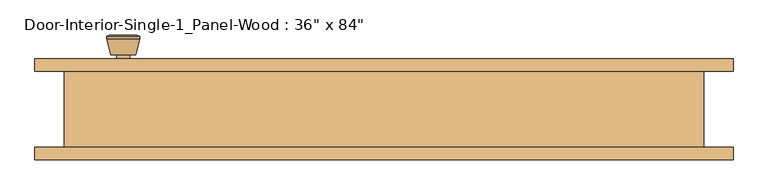
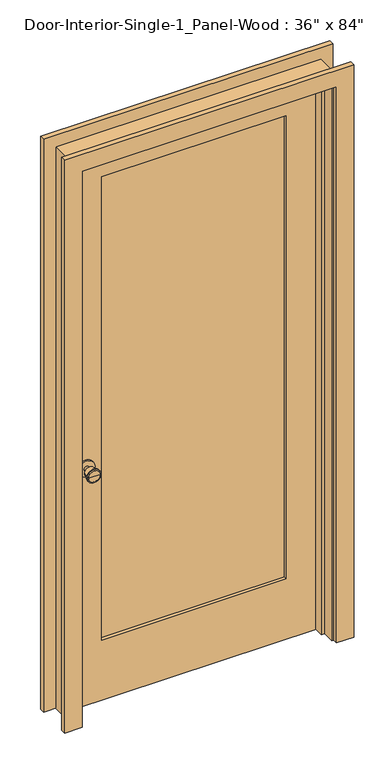
"""IFC4 building model written with IfcOpenShell, lengths in millimetres: door geometry."""

from ifc_helpers import new_model, si_unit, point, frame, frame_2d, origin, place, context, project, spatial, polyline, circle_curve, trimmed, segment, composite_curve, outline, extrude, faceted_brep, source, transform, mapped, element, save
from ifc_brep_helpers import plane_surface, cylinder_surface, revolved_surface, advanced_brep


def door_3c6ab76a(model_context):
    return source(origin(), model_context, "Body", "SolidModel", [
        advanced_brep(
        [(-393.7, 13.05, 914.4), (-383.7, 13.05, 914.4), (-403.7, 13.05, 914.4), (-373.2241324, -35.95, 914.4), (-393.7, -35.95, 914.4), (-414.1758676, -35.95, 914.4), (-368.7, -34.1221319, 914.4), (-418.7, -34.1221319, 914.4), (-368.7, -30.6584537, 914.4), (-418.7, -30.6584537, 914.4), (-375.063764, -5.95, 914.4), (-412.336236, -5.95, 914.4), (-383.7, -5.95, 914.4), (-403.7, -5.95, 914.4)],
        [
            (0, 1),
            (1, 2, circle_curve(frame((-393.7, 13.05, 914.4), z_axis=(0.0, 1.0, 0.0), x_axis=(-1.0, 0.0, 0.0)), 10.0)),
            (2, 0),
            (2, 1, circle_curve(frame((-393.7, 13.05, 914.4), z_axis=(0.0, 1.0, 0.0), x_axis=(-1.0, 0.0, 0.0)), 10.0)),
            (3, 4),
            (4, 5),
            (5, 3, circle_curve(frame((-393.7, -35.95, 914.4), z_axis=(0.0, -1.0, 0.0), x_axis=(-1.0, 0.0, 0.0)), 20.4758676)),
            (3, 5, circle_curve(frame((-393.7, -35.95, 914.4), z_axis=(0.0, -1.0, 0.0), x_axis=(-1.0, 0.0, 0.0)), 20.4758676)),
            (6, 3),
            (5, 7),
            (7, 6, circle_curve(frame((-393.7, -34.1221319, 914.4), z_axis=(0.0, -1.0, 0.0), x_axis=(-1.0, 0.0, 0.0)), 25.0)),
            (6, 7, circle_curve(frame((-393.7, -34.1221319, 914.4), z_axis=(0.0, -1.0, 0.0), x_axis=(-1.0, 0.0, 0.0)), 25.0)),
            (8, 6),
            (7, 9),
            (9, 8, circle_curve(frame((-393.7, -30.6584537, 914.4), z_axis=(0.0, -1.0, 0.0), x_axis=(-1.0, 0.0, 0.0)), 25.0)),
            (8, 9, circle_curve(frame((-393.7, -30.6584537, 914.4), z_axis=(0.0, -1.0, 0.0), x_axis=(-1.0, 0.0, 0.0)), 25.0)),
            (10, 8),
            (9, 11),
            (11, 10, circle_curve(frame((-393.7, -5.95, 914.4), z_axis=(0.0, -1.0, 0.0), x_axis=(-1.0, 0.0, 0.0)), 18.636236)),
            (10, 11, circle_curve(frame((-393.7, -5.95, 914.4), z_axis=(0.0, -1.0, 0.0), x_axis=(-1.0, 0.0, 0.0)), 18.636236)),
            (12, 10),
            (11, 13),
            (13, 12, circle_curve(frame((-393.7, -5.95, 914.4), z_axis=(0.0, -1.0, 0.0), x_axis=(-1.0, 0.0, 0.0)), 10.0)),
            (12, 13, circle_curve(frame((-393.7, -5.95, 914.4), z_axis=(0.0, -1.0, 0.0), x_axis=(-1.0, 0.0, 0.0)), 10.0)),
            (1, 12),
            (13, 2),
        ],
        [
            plane_surface(frame((-393.7, 13.05, 914.4), z_axis=(0.0, 1.0, 0.0), x_axis=(-1.0, 0.0, 0.0))),
            plane_surface(frame((-393.7, -35.95, 914.4), z_axis=(0.0, -1.0, 0.0), x_axis=(-1.0, 0.0, 0.0))),
            revolved_surface(polyline([(-414.1758676, -35.95, 914.4), (-418.7, -34.1221319, 914.4)]), (-393.7, 13.05, 914.4), (0.0, 1.0, 0.0)),
            cylinder_surface(frame((-393.7, 13.05, 914.4), z_axis=(0.0, 1.0, 0.0), x_axis=(-1.0, 0.0, 0.0)), 25.0),
            revolved_surface(polyline([(-418.7, -30.6584537, 914.4), (-412.336236, -5.95, 914.4)]), (-393.7, 13.05, 914.4), (0.0, 1.0, 0.0)),
            plane_surface(frame((-393.7, -5.95, 914.4), z_axis=(0.0, 1.0, 0.0), x_axis=(-1.0, 0.0, 0.0))),
            cylinder_surface(frame((-393.7, 13.05, 914.4), z_axis=(0.0, 1.0, 0.0), x_axis=(-1.0, 0.0, 0.0)), 10.0),
        ],
        [
            (0, [[1, 2, 3]]),
            (0, [[-3, 4, -1]]),
            (1, [[5, 6, 7]]),
            (1, [[-6, -5, 8]]),
            (2, [[9, -7, 10, 11]]),
            (2, [[-10, -8, -9, 12]]),
            (3, [[13, -11, 14, 15]]),
            (3, [[-14, -12, -13, 16]]),
            (4, [[17, -15, 18, 19]]),
            (4, [[-18, -16, -17, 20]]),
            (5, [[21, -19, 22, 23]]),
            (5, [[-22, -20, -21, 24]]),
            (6, [[25, -23, 26, -2]]),
            (6, [[-26, -24, -25, -4]]),
        ],
    ),
        extrude(outline(composite_curve([segment(trimmed(circle_curve(frame_2d((914.4, -393.7)), 30.0), [point((914.4, -423.7))], [point((914.4, -363.7))], False, "CARTESIAN"), True, "CONTINUOUS"), segment(trimmed(circle_curve(frame_2d((914.4, -393.7)), 30.0), [point((914.4, -363.7))], [point((914.4, -423.7))], False, "CARTESIAN"), True, "CONTINUOUS")], self_intersect=False)), frame((0.0, 13.05, 0.0), z_axis=(0.0, 1.0, 0.0), x_axis=(0.0, 0.0, 1.0)), (0.0, 0.0, 1.0), 6.0),
        advanced_brep(
        [(-393.7, 59.975, 914.4), (-403.7, 59.975, 914.4), (-383.7, 59.975, 914.4), (-373.2241324, 108.975, 914.4), (-414.1758676, 108.975, 914.4), (-393.7, 108.975, 914.4), (-368.7, 107.1471319, 914.4), (-418.7, 107.1471319, 914.4), (-368.7, 103.6834537, 914.4), (-418.7, 103.6834537, 914.4), (-375.063764, 78.975, 914.4), (-412.336236, 78.975, 914.4), (-383.7, 78.975, 914.4), (-403.7, 78.975, 914.4)],
        [
            (0, 1),
            (1, 2, circle_curve(frame((-393.7, 59.975, 914.4), z_axis=(0.0, -1.0, 0.0), x_axis=(-1.0, 0.0, 0.0)), 10.0)),
            (2, 0),
            (2, 1, circle_curve(frame((-393.7, 59.975, 914.4), z_axis=(0.0, -1.0, 0.0), x_axis=(-1.0, 0.0, 0.0)), 10.0)),
            (3, 4, circle_curve(frame((-393.7, 108.975, 914.4), z_axis=(0.0, 1.0, 0.0), x_axis=(-1.0, 0.0, 0.0)), 20.4758676)),
            (4, 5),
            (5, 3),
            (4, 3, circle_curve(frame((-393.7, 108.975, 914.4), z_axis=(0.0, 1.0, 0.0), x_axis=(-1.0, 0.0, 0.0)), 20.4758676)),
            (6, 7, circle_curve(frame((-393.7, 107.1471319, 914.4), z_axis=(0.0, 1.0, 0.0), x_axis=(-1.0, 0.0, 0.0)), 25.0)),
            (7, 4),
            (3, 6),
            (7, 6, circle_curve(frame((-393.7, 107.1471319, 914.4), z_axis=(0.0, 1.0, 0.0), x_axis=(-1.0, 0.0, 0.0)), 25.0)),
            (8, 9, circle_curve(frame((-393.7, 103.6834537, 914.4), z_axis=(0.0, 1.0, 0.0), x_axis=(-1.0, 0.0, 0.0)), 25.0)),
            (9, 7),
            (6, 8),
            (9, 8, circle_curve(frame((-393.7, 103.6834537, 914.4), z_axis=(0.0, 1.0, 0.0), x_axis=(-1.0, 0.0, 0.0)), 25.0)),
            (10, 11, circle_curve(frame((-393.7, 78.975, 914.4), z_axis=(0.0, 1.0, 0.0), x_axis=(-1.0, 0.0, 0.0)), 18.636236)),
            (11, 9),
            (8, 10),
            (11, 10, circle_curve(frame((-393.7, 78.975, 914.4), z_axis=(0.0, 1.0, 0.0), x_axis=(-1.0, 0.0, 0.0)), 18.636236)),
            (12, 13, circle_curve(frame((-393.7, 78.975, 914.4), z_axis=(0.0, 1.0, 0.0), x_axis=(-1.0, 0.0, 0.0)), 10.0)),
            (13, 11),
            (10, 12),
            (13, 12, circle_curve(frame((-393.7, 78.975, 914.4), z_axis=(0.0, 1.0, 0.0), x_axis=(-1.0, 0.0, 0.0)), 10.0)),
            (1, 13),
            (12, 2),
        ],
        [
            plane_surface(frame((-393.7, 59.975, 914.4), z_axis=(0.0, -1.0, 0.0), x_axis=(-1.0, 0.0, 0.0))),
            plane_surface(frame((-393.7, 108.975, 914.4), z_axis=(0.0, 1.0, 0.0), x_axis=(-1.0, 0.0, 0.0))),
            revolved_surface(polyline([(-414.1758676, 108.975, 914.4), (-418.7, 107.1471319, 914.4)]), (-393.7, 59.975, 914.4), (0.0, -1.0, 0.0)),
            cylinder_surface(frame((-393.7, 59.975, 914.4), z_axis=(0.0, -1.0, 0.0), x_axis=(-1.0, 0.0, 0.0)), 25.0),
            revolved_surface(polyline([(-418.7, 103.6834537, 914.4), (-412.336236, 78.975, 914.4)]), (-393.7, 59.975, 914.4), (0.0, -1.0, 0.0)),
            plane_surface(frame((-393.7, 78.975, 914.4), z_axis=(0.0, -1.0, 0.0), x_axis=(-1.0, 0.0, 0.0))),
            cylinder_surface(frame((-393.7, 59.975, 914.4), z_axis=(0.0, -1.0, 0.0), x_axis=(-1.0, 0.0, 0.0)), 10.0),
        ],
        [
            (0, [[1, 2, 3]]),
            (0, [[-3, 4, -1]]),
            (1, [[5, 6, 7]]),
            (1, [[8, -7, -6]]),
            (2, [[9, 10, -5, 11]]),
            (2, [[12, -11, -8, -10]]),
            (3, [[13, 14, -9, 15]]),
            (3, [[16, -15, -12, -14]]),
            (4, [[17, 18, -13, 19]]),
            (4, [[20, -19, -16, -18]]),
            (5, [[21, 22, -17, 23]]),
            (5, [[24, -23, -20, -22]]),
            (6, [[-2, 25, -21, 26]]),
            (6, [[-4, -26, -24, -25]]),
        ],
    ),
        extrude(outline(composite_curve([segment(trimmed(circle_curve(frame_2d((914.4, -393.7)), 30.0), [point((914.4, -423.7))], [point((914.4, -363.7))], False, "CARTESIAN"), True, "CONTINUOUS"), segment(trimmed(circle_curve(frame_2d((914.4, -393.7)), 30.0), [point((914.4, -363.7))], [point((914.4, -423.7))], False, "CARTESIAN"), True, "CONTINUOUS")], self_intersect=False)), frame((0.0, 53.975, 0.0), z_axis=(0.0, 1.0, 0.0), x_axis=(0.0, 0.0, 1.0)), (0.0, 0.0, 1.0), 6.0),
        faceted_brep([(482.6, 53.975, 0.0), (482.6, -60.325, 0.0), (457.2, -60.325, 0.0), (457.2, -15.875, 0.0), (444.5, -15.875, 0.0), (444.5, 19.05, 0.0), (457.2, 19.05, 0.0), (457.2, 53.975, 0.0), (482.6, 53.975, 2159.0), (482.6, -60.325, 2159.0), (-482.6, -60.325, 2159.0), (-482.6, -60.325, 0.0), (-457.2, -60.325, 0.0), (-457.2, -60.325, 2133.6), (457.2, -60.325, 2133.6), (457.2, -15.875, 2133.6), (-457.2, -15.875, 2133.6), (-457.2, -15.875, 0.0), (-444.5, -15.875, 0.0), (-444.5, -15.875, 2120.9), (444.5, -15.875, 2120.9), (444.5, 19.05, 2120.9), (-444.5, 19.05, 2120.9), (-444.5, 19.05, 0.0), (-457.2, 19.05, 0.0), (-457.2, 19.05, 2133.6), (457.2, 19.05, 2133.6), (457.2, 53.975, 2133.6), (-457.2, 53.975, 2133.6), (-457.2, 53.975, 0.0), (-482.6, 53.975, 0.0), (-482.6, 53.975, 2159.0)], [[[0, 1, 2, 3, 4, 5, 6, 7]], [[1, 0, 8, 9]], [[2, 1, 9, 10, 11, 12, 13, 14]], [[3, 2, 14, 15]], [[4, 3, 15, 16, 17, 18, 19, 20]], [[5, 4, 20, 21]], [[6, 5, 21, 22, 23, 24, 25, 26]], [[7, 6, 26, 27]], [[0, 7, 27, 28, 29, 30, 31, 8]], [[9, 8, 31, 10]], [[15, 14, 13, 16]], [[21, 20, 19, 22]], [[27, 26, 25, 28]], [[30, 29, 24, 23, 18, 17, 12, 11]], [[10, 31, 30, 11]], [[16, 13, 12, 17]], [[22, 19, 18, 23]], [[28, 25, 24, 29]]]),
        extrude(outline(polyline([(2133.6, -457.2), (0.0, -457.2), (0.0, 457.2), (2133.6, 457.2), (2133.6, -457.2)]), holes=[polyline([(2014.5375, -336.55), (2014.5375, 336.55), (231.775, 336.55), (231.775, -336.55), (2014.5375, -336.55)])]), frame((0.0, 19.05, 0.0), z_axis=(0.0, 1.0, 0.0), x_axis=(0.0, 0.0, 1.0)), (0.0, 0.0, 1.0), 34.925),
        extrude(outline(polyline([(336.55, 30.6916667), (-336.55, 30.6916667), (-336.55, 42.3333333), (336.55, 42.3333333), (336.55, 30.6916667)])), frame((0.0, 0.0, 231.775), z_axis=(0.0, 0.0, 1.0), x_axis=(1.0, 0.0, 0.0)), (0.0, 0.0, 1.0), 1782.7625),
        extrude(outline(polyline([(0.0, 463.55), (0.0, 527.05), (2203.45, 527.05), (2203.45, -527.05), (0.0, -527.05), (0.0, -463.55), (2139.95, -463.55), (2139.95, 463.55), (0.0, 463.55)])), frame((0.0, 53.975, 0.0), z_axis=(0.0, 1.0, 0.0), x_axis=(0.0, 0.0, 1.0)), (0.0, 0.0, 1.0), 19.05),
        extrude(outline(polyline([(0.0, 463.55), (0.0, 527.05), (2203.45, 527.05), (2203.45, -527.05), (0.0, -527.05), (0.0, -463.55), (2139.95, -463.55), (2139.95, 463.55), (0.0, 463.55)])), frame((0.0, -79.375, 0.0), z_axis=(0.0, 1.0, 0.0), x_axis=(0.0, 0.0, 1.0)), (0.0, 0.0, 1.0), 19.05),
    ])


if __name__ == "__main__":
    model = new_model("IFC4")
    model_context = context("Model", 3, world=origin())
    ifc_project = project(units=[si_unit("LENGTHUNIT", "METRE", prefix="MILLI")], contexts=[model_context])
    site = spatial("IfcSite", under=ifc_project)
    building = spatial("IfcBuilding", under=site)
    placement = place(None, origin())
    door_shape = door_3c6ab76a(model_context)
    element("IfcDoor", 1, ObjectType="Door-Interior-Single-1_Panel-Wood : 36\" x 84\"", at=placement, inside=building, context=model_context, shape_type="MappedRepresentation", body=[
        mapped(door_shape, transform((0.0, 0.0, 0.0), x_axis=(1.0, 0.0, 0.0), y_axis=(0.0, 1.0, 0.0), z_axis=(0.0, 0.0, 1.0))),
    ])
    save(model, "model.ifc")

# Revit data of these elements
# Type "Door-Interior-Single-1_Panel-Wood : 36\" x 84\""
#   Type Mark = "8"
#   Assembly Code = "C1020300"
#   Analytic Construction = "Wooden"
#   Top Rail = 0' - 4 11/16"
#   Thickness = 0' - 1 3/8"
#   Thermal Resistance (R) = 2.5876 (h·ft²·°F)/BTU
#   Swing Angle [instance default] = 90.00°
#   Stiles = 0' - 4 3/4"
#   Rough Width = 3' - 2"
#   Rough Height = 7' - 1"
#   Height = 7' - 0"
#   Width = 3' - 0"
#   Heat Transfer Coefficient (U) = 0.3865 BTU/(h·ft²·°F)
#   Bottom Rail = 0' - 9 1/8"
#   Trim Material = Cherry
#   Panel Material = Cherry
#   Frame Material = Cherry
#   Door Handle Material = Aluminum
#   Visual Light Transmittance = 0
#   Solar Heat Gain Coefficient = 0
#   Wall Closure = (empty or 0)
#   Function = (empty or 0)
# Element 1 (IfcDoor, "Door-Interior-Single-1_Panel-Wood : 36\" x 84\"")
#   Materials on its faces: "Cherry", "Aluminum"
# Materials
#   "Cherry": class "Wood", colour RGB 226 177 128, transparency 0, Description = "Prunus Serotina", Cost = 0
#   "Aluminum": class "Metal", colour RGB 247 247 247, transparency 0, Description = "Aluminum 6061", Cost = 0
